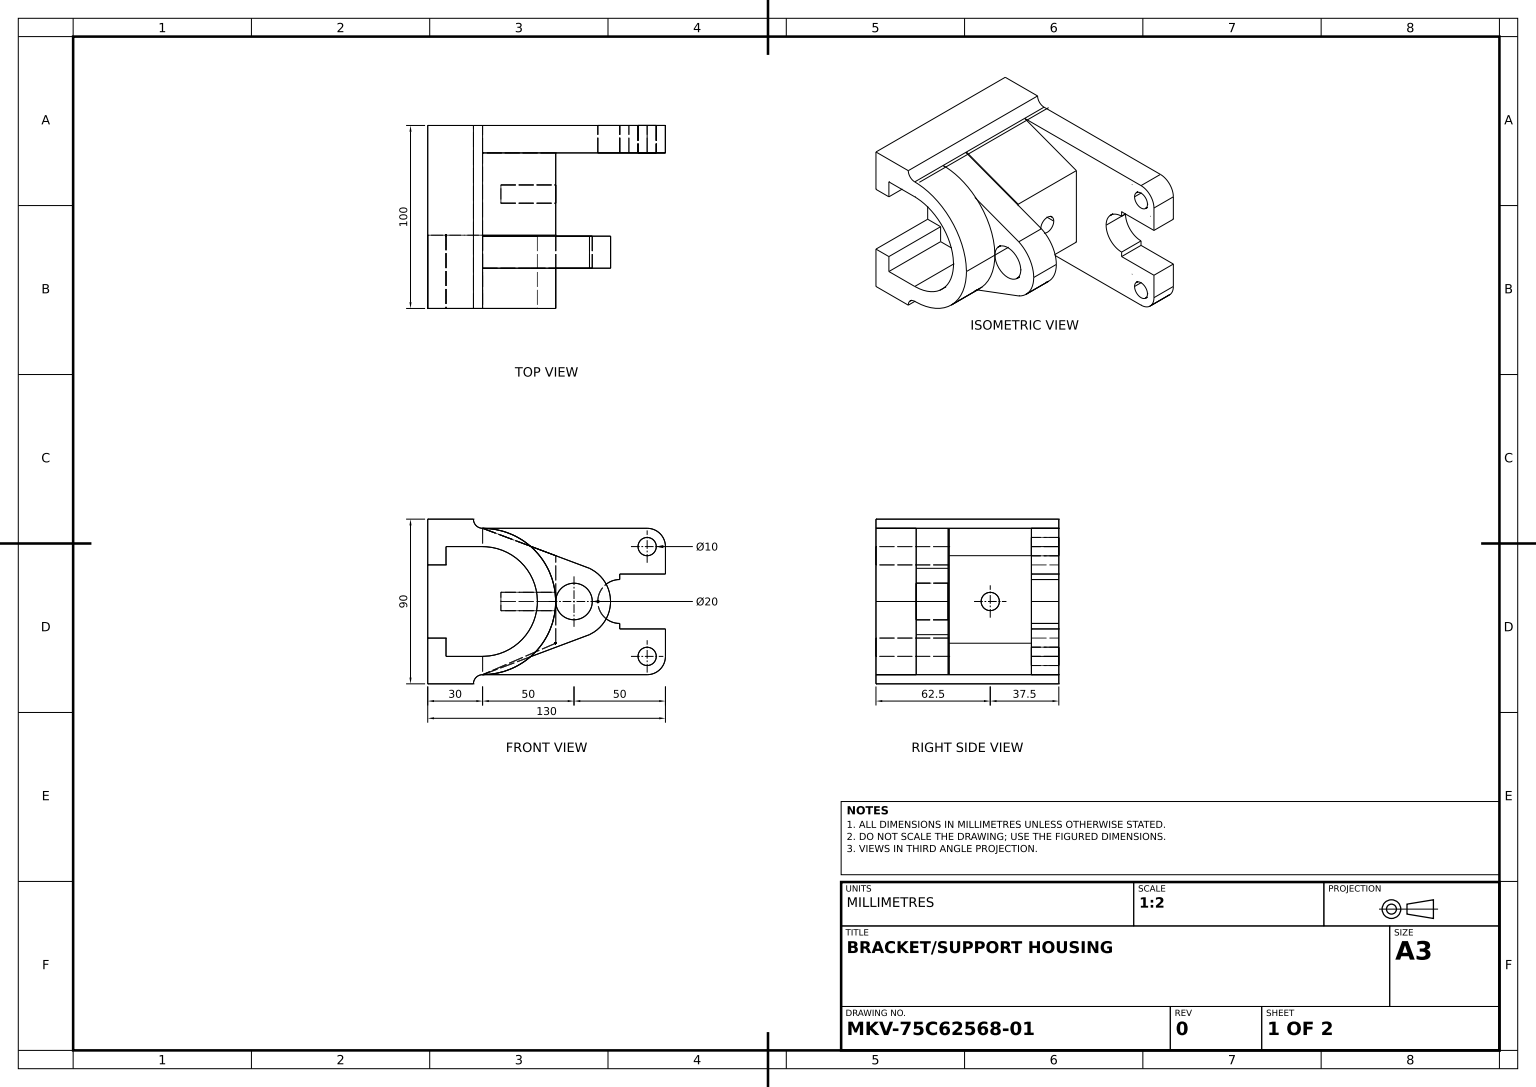
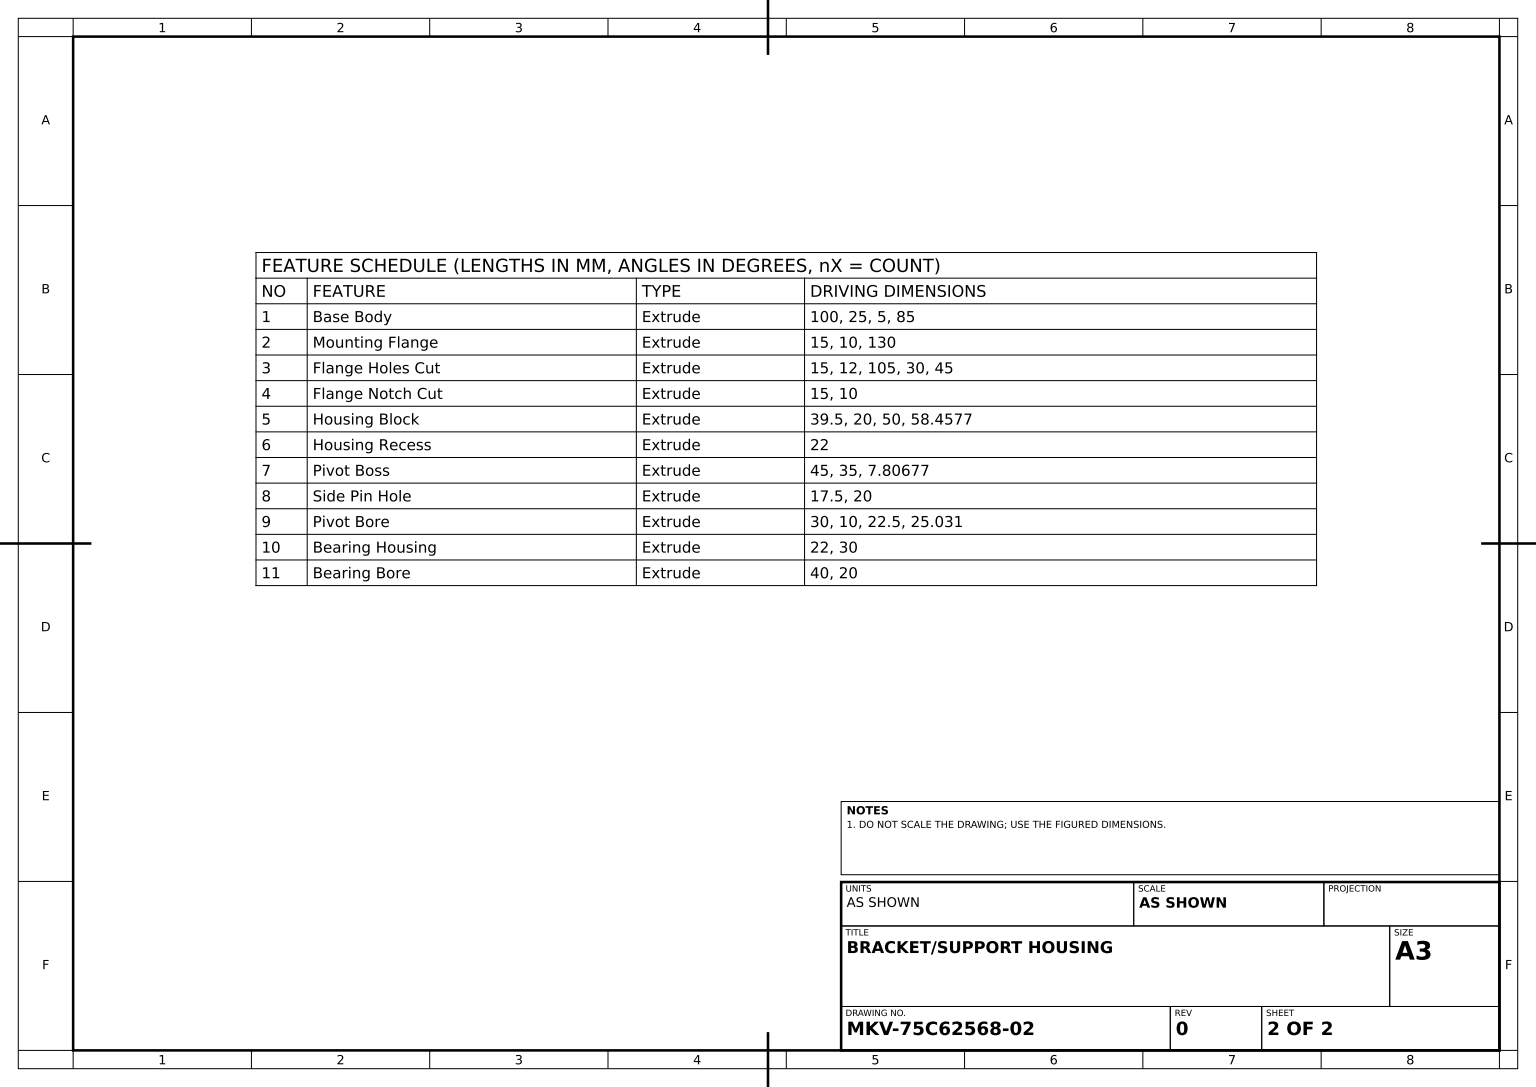
SolidWorks part; units mm, degrees
material "Plain Carbon Steel"
ref_plane "Front Plane" through (0, 0, 0) normal (0, 0, 1) x (1, 0, 0)
ref_plane "Top Plane" through (0, 0, 0) normal (0, 1, 0) x (1, 0, 0)
ref_plane "Right Plane" through (0, 0, 0) normal (1, 0, 0) x (0, 0, -1)
sketch "Base Body Profile" plane through (0, 0, 0) normal (0, 0, 1) x (1, 0, 0)
  line L0 (0, 0) -> (0, 90)
  line L1 (0, 90) -> (25, 90)
  line L2 (30, 85) -> (30, 5)
  line L3 (25, 0) -> (0, 0)
  arc A0 (25, 90) -> (30, 85) centre (30, 90) ccw
  arc A1 (30, 5) -> (25, 0) centre (30, 0) ccw
  dimension "D1" = 25
  dimension "D2" = 5
  dimension "D3" = 85
extrude "Base Body" add sketch "Base Body Profile" along normal blind 100
sketch "Mounting Flange Profile" plane through (0, 0, 0) normal (0, 0, -1) x (-1, 0, 0)
  line L0 (0, 90) -> (0, 0) construction
  line L2 (-130, 45) -> (-130, 75)
  line L4 (-130, 45) -> (-130, 15)
  line L6 (-120, 85) -> (-30, 85)
  line L7 (-30, 85) -> (-30, 5)
  line L8 (-30, 5) -> (-120, 5)
  arc A0 (-120, 85) -> (-130, 75) centre (-120, 75) ccw
  arc A1 (-130, 15) -> (-120, 5) centre (-120, 15) ccw
  dimension "D1" = 10
  dimension "D2" = 130
extrude "Mounting Flange" add sketch "Mounting Flange Profile" against normal blind 15
sketch "Flange Holes Profile" plane through (0, 0, 0) normal (0, 0, -1) x (-1, 0, 0)
  line L0 (-130, 60) -> (-130, 30)
  line L1 (-130, 75) -> (-130, 15) construction
  line L5 (0, 90) -> (0, 0) construction
  line L6 (-105, 60) -> (-130, 60)
  line L7 (0, 0) -> (-25, 0) construction
  line L9 (-105, 30) -> (-130, 30)
  line L10 (-105, 60) -> (-105, 57)
  line L11 (-105, 33) -> (-105, 30)
  arc A0 (-105, 33) -> (-105, 57) centre (-105, 45) ccw
  dimension "D1" = 12
  dimension "D2" = 105
  dimension "D3" = 30
  dimension "D4" = 45
extrude "Flange Holes Cut" cut sketch "Flange Holes Profile" against normal blind 15
sketch "Flange Notch Profile" plane through (0, 0, 15) normal (0, 0, 1) x (1, 0, 0)
  circle A0 centre (120, 75) radius 5
  circle A1 centre (120, 15) radius 5
  dimension "D1" = 10
extrude "Flange Notch Cut" cut sketch "Flange Notch Profile" against normal blind 15
sketch "Housing Block Profile" plane through (0, 0, 100) normal (0, 0, 1) x (1, 0, 0)
  line L0 (30, 5) -> (30, 85) construction
  line L2 (30, 85) -> (88.4577, 63.1237)
  line L3 (30, 85) -> (30, 5)
  line L4 (30, 5) -> (88.4577, 26.8763)
  arc A0 (88.4577, 26.8763) -> (88.4577, 63.1237) centre (80, 45) ccw
  dimension "D1" = 20
  dimension "D2" = 50
  dimension "D3" = 58.4577
extrude "Housing Block" add sketch "Housing Block Profile" against normal blind 39.5
sketch "Housing Recess Profile" plane through (0, 0, 100) normal (0, 0, 1) x (1, 0, 0)
  line L0 (30, 85) -> (30, 5)
  line L1 (30, 5) -> (88.4577, 26.8763)
  line L3 (88.4577, 63.1237) -> (30, 85)
  arc A0 (88.4577, 26.8763) -> (88.4577, 63.1237) centre (80, 45) ccw
extrude "Housing Recess" cut sketch "Housing Recess Profile" against normal blind 22
sketch "Pivot Boss Profile" plane through (0, 0, 15) normal (0, 0, 1) x (1, 0, 0)
  line L0 (30, 85) -> (30, 5)
  line L1 (30, 45) -> (70, 45)
  line L2 (70, 45) -> (70, 70.031)
  line L3 (88.4577, 63.1237) -> (30, 85) construction
  line L4 (70, 70.031) -> (30, 85)
  line L5 (70, 45) -> (70, 22.1932)
  line L6 (70, 22.1932) -> (30, 5)
  line L7 (105, 30) -> (105, 33) construction
  line L8 (130, 30) -> (105, 30) construction
  line M12 (30, 85) -> (30, 5)
  dimension "D1" = 35
  dimension "D2" = 7.8068
extrude "Pivot Boss" add sketch "Pivot Boss Profile" along normal blind 45 contours L2 L4 L1 M12 | L6 L5 L1 L0
sketch "Side Pin Hole Profile" plane through (0, 0, 78) normal (0, 0, 1) x (1, 0, 0)
  circle A0 centre (80, 45) radius 10
  dimension "D1" = 20
extrude "Side Pin Hole" cut sketch "Side Pin Hole Profile" against normal blind 17.5
sketch "Pivot Bore Profile" plane through (70, 0, 0) normal (1, 0, 0) x (0, 0, -1)
  line L0 (-15, 22.1932) -> (-15, 70.031) construction
  line L1 (-60, 70.031) -> (-15, 70.031) construction
  circle A0 centre (-37.5, 45) radius 5
  dimension "D1" = 10
  dimension "D2" = 22.5
  dimension "D3" = 25.031
extrude "Pivot Bore" cut sketch "Pivot Bore Profile" against normal blind 30
sketch "Bearing Housing Profile" plane through (0, 0, 100) normal (0, 0, 1) x (1, 0, 0)
  line L0 (30, 85) -> (30, 5) construction
  line L1 (30, 75) -> (10, 75)
  line L2 (10, 75) -> (10, 65)
  line L3 (10, 65) -> (0, 65)
  line L4 (0, 90) -> (0, 0) construction
  line L5 (30, 15) -> (10, 15)
  line L6 (10, 15) -> (10, 25)
  line L7 (30, 85) -> (30, 75)
  line L8 (10, 25) -> (0, 25)
  line L9 (30, 85) -> (30, 75)
  line L10 (30, 5) -> (30, 15)
  arc A0 (30, 5) -> (30, 85) centre (30, 45) ccw
  arc A1 (30, 15) -> (30, 75) centre (30, 45) ccw
  line M1 (30, 5) -> (30, 85)
  dimension "D1" = 30
extrude "Bearing Housing" add sketch "Bearing Housing Profile" against normal blind 22 contours A1 A0 M1
sketch "Bearing Bore Profile" plane through (0, 0, 100) normal (0, 0, 1) x (1, 0, 0)
  line L0 (30, 75) -> (30, 15) construction
  line L1 (30, 75) -> (10, 75)
  line L2 (30, 75) -> (30, 15) construction
  line L4 (10, 75) -> (10, 65)
  line L5 (10, 65) -> (0, 65)
  line L6 (0, 90) -> (0, 0) construction
  line L7 (30, 15) -> (10, 15)
  line L10 (10, 15) -> (10, 25)
  line L11 (10, 25) -> (0, 25)
  line L12 (0, 25) -> (0, 65)
  arc A1 (30, 15) -> (30, 75) centre (30, 45) ccw
  dimension "D1" = 20
extrude "Bearing Bore" cut sketch "Bearing Bore Profile" against normal blind 40
